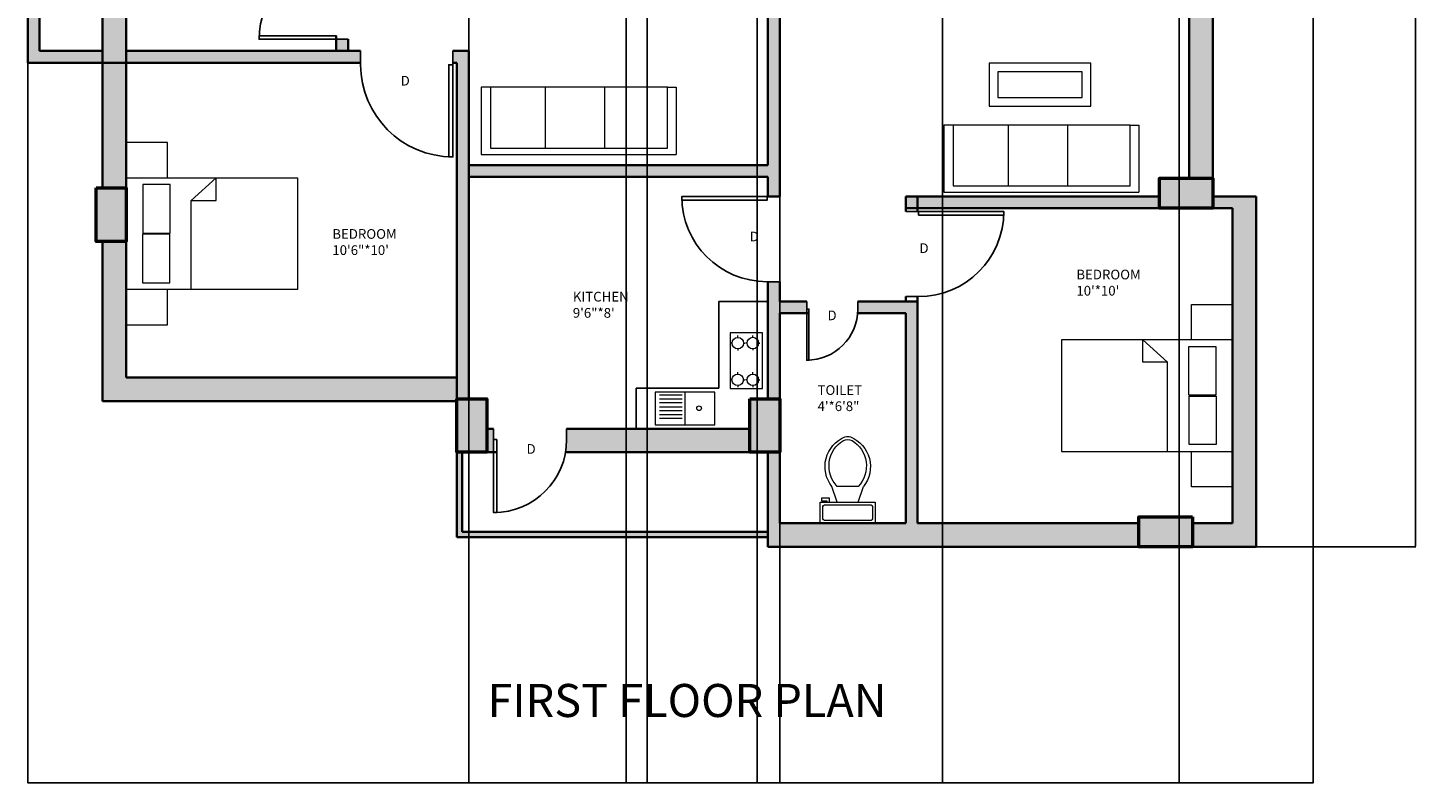
# Model space of a CAD drawing. Units: inches. Extents: x 1998 to 2588, y 1139 to 1977.
# Tile 1 of 134: x 2059 to 2588, y 1139 to 1427. Entities that reach past the tile are written whole.
import ezdxf

# ---------------------------------------------------------------- set-up
doc = ezdxf.new("R2010")
doc.units = ezdxf.units.IN
for name, color, linetype, lineweight in [('A-ANNO-DIMS', 2, 'Continuous', 18), ('A-ANNO-TITL', 7, 'Continuous', 35), ('A-AREA-IDEN', 7, 'Continuous', 18), ('A-COLS-PATT', 250, 'Continuous', 13), ('A-DOOR-IDEN', 7, 'Continuous', 18), ('A-EQPM', 21, 'Continuous', 18), ('A-FLOR-CASE', 32, 'Continuous', 25), ('A-FLOR-FIXT', 9, 'Continuous', 18), ('A-WALL-PATT', 252, 'Continuous', 13), ('COLUMN', 10, 'Continuous', 50), ('DOOR', 52, 'Continuous', 25), ('FUR', 21, 'Continuous', 18), ('WALL', 200, 'Continuous', 35)]:
    doc.layers.add(name, color=color, linetype=linetype, lineweight=lineweight)
doc.styles.get("Standard").update_dxf_attribs({"font": 'arial.ttf'})
doc.dimstyles.get("Standard").update_dxf_attribs({"dimtxt": 0.18, "dimasz": 0.18, "dimexe": 0.18, "dimexo": 0.0625, "dimgap": 0.09, "dimtad": 0, "dimtih": 1, "dimtoh": 1, "dimdec": 4, "dimzin": 0, "dimdsep": 46, "dimtxsty": 'Standard', "dimcen": 0.09, "dimadec": 0, "dimazin": 0, "dimtfac": 1, "dimtdec": 4, "dimtofl": 0, "dimtmove": 0, "dimatfit": 3, "dimfxl": 1, "dimtolj": 1, "dimtzin": 0, "dimarcsym": 0})

# ---------------------------------------------------------------- blocks, each defined once
blk = doc.blocks.new('*U2')
for p, q in [((0, 0), (0, -6)), ((40, 0), (40, -6))]:
    blk.add_line(p, q)
blk.add_lwpolyline([(0, 0), (0, 40), (1.75, 40), (1.75, 0)], close=True)
blk.add_arc((0, 0), 40, 0, 90)
blk = doc.blocks.new('*U4')
for p, q in [((9.5, -6), (9.5, -2)), ((-10, -8.5), (-8, -8.5)), ((-10, -9.5), (-10, -8.5)), ((-7, -9.5), (-10, -9.5)), ((-8, -8.5), (-8, -8)), ((-7, -8), (-7, -9.5)), ((-4, -8), (-6, -14)), ((4, -8), (6, -14)), ((4, -14), (-4, -14))]:
    blk.add_line(p, q)
blk.add_lwpolyline([(10.5, -8), (10.5, 0), (-10.5, 0), (-10.5, -8)], close=True)
for points in [[(-9.5, -2), (-9.5, -6)], [(8.5, -1), (-8.5, -1)], [(-8.5, -7), (8.5, -7)]]:
    blk.add_lwpolyline(points)
for centre, radius, start, end in [((-8.62, -1.88), 0.884, 81.8699, 188.1301), ((8.62, -1.88), 0.884, 351.8699, 98.1301), ((-8.62, -6.12), 0.884, 171.8699, 278.1301), ((8.62, -6.12), 0.884, 261.8699, 8.1301), ((3.52, -21.58), 12.17, 141.4691, 247.9714), ((4.2, -21.82), 11.33, 136.3677, 238.9468), ((-3.52, -21.58), 12.17, 292.0284, 38.5307), ((-4.2, -21.82), 11.33, 301.053, 43.6321), ((0, -27.88), 4, 245.7318, 294.2682), ((0, -29), 4, 254.8605, 285.1395)]:
    blk.add_arc(centre, radius, start, end)
blk = doc.blocks.new('BED-WITH-NIGHTSTANDS')
for p, q in [((34.22, 56), (24.8, 47.44)), ((34.22, 47.44), (34.22, 56)), ((24.8, 13.42), (24.8, 47.44)), ((24.8, 47.44), (34.22, 47.44))]:
    blk.add_line(p, q)
for points in [[(0, 56), (15.7, 56), (15.7, 69.42), (0, 69.42)], [(0, 56), (65.22, 56), (65.22, 13.42), (0, 13.42)], [(6.37, 34.93), (16.73, 34.93), (16.73, 53.45), (6.37, 53.45)], [(6.25, 16.05), (16.6, 16.05), (16.6, 34.57), (6.25, 34.57)], [(0, 0), (15.7, 0), (15.7, 13.42), (0, 13.42)]]:
    blk.add_lwpolyline(points, close=True)
blk = doc.blocks.new('SOFA-THREE-SEAT')
for p, q in [((3.6, 25.61), (0, 25.61)), ((0, 25.61), (0, 0)), ((24.45, 25.61), (24.45, 2.42)), ((47.08, 25.61), (47.08, 2.42)), ((71.01, 25.61), (74.34, 25.61)), ((74.34, 25.61), (74.34, 0)), ((0, 0), (74.34, 0))]:
    blk.add_line(p, q)
blk.add_lwpolyline([(3.6, 2.42), (71.01, 2.42), (71.01, 25.61), (3.6, 25.61)], close=True)
blk = doc.blocks.new('TABLE-COFFEE')
for points in [[(0, 0), (38.73, 0), (38.73, 16.33), (0, 16.33)], [(3.28, 3.28), (35.45, 3.28), (35.45, 13.05), (3.28, 13.05)]]:
    blk.add_lwpolyline(points, close=True)
blk = doc.blocks.new('*D23')
at = {"layer": 'A-ANNO-DIMS', "color": 0, "lineweight": -2, "transparency": 16777216}
for p, q in [((2549.18, 1476.17), (2549.18, 1138.6)), ((2059.47, 1413.17), (2059.47, 1138.6)), ((2059.65, 1138.78), (2303.93, 1138.78)), ((2549, 1138.78), (2304.72, 1138.78))]:
    blk.add_line(p, q, dxfattribs=at)
at = {"layer": 'A-ANNO-DIMS', "color": 0, "transparency": 16777216}
for points in [[(2059.65, 1138.81), (2059.65, 1138.75), (2059.47, 1138.78)], [(2549, 1138.81), (2549, 1138.75), (2549.18, 1138.78)]]:
    blk.add_solid(points, dxfattribs=at)
at = {"layer": 'Defpoints', "color": 0, "transparency": 16777216}
for p in [(2549.18, 1476.23), (2059.47, 1413.23), (2549.18, 1138.78)]:
    blk.add_point(p, dxfattribs=at)
at = {"layer": 'A-ANNO-DIMS', "color": 0, "transparency": 16777216, "insert": (2304.33, 1138.78), "char_height": 0.18, "attachment_point": 5}
blk.add_mtext('\\A1;489.7', dxfattribs=at)
blk = doc.blocks.new('*D24')
at = {"layer": 'A-ANNO-DIMS', "color": 0, "lineweight": -2, "transparency": 16777216}
for p, q in [((2398.54, 1911.23), (2588.31, 1911.23)), ((2588.13, 1911.05), (2588.13, 1570.16)), ((2588.13, 1228.91), (2588.13, 1569.8)), ((2527.54, 1228.73), (2588.31, 1228.73))]:
    blk.add_line(p, q, dxfattribs=at)
at = {"layer": 'A-ANNO-DIMS', "color": 0, "transparency": 16777216}
for points in [[(2588.1, 1911.05), (2588.16, 1911.05), (2588.13, 1911.23)], [(2588.1, 1228.91), (2588.16, 1228.91), (2588.13, 1228.73)]]:
    blk.add_solid(points, dxfattribs=at)
at = {"layer": 'Defpoints', "color": 0, "transparency": 16777216}
for p in [(2398.47, 1911.23), (2588.13, 1911.23), (2527.47, 1228.73)]:
    blk.add_point(p, dxfattribs=at)
at = {"layer": 'A-ANNO-DIMS', "color": 0, "transparency": 16777216, "insert": (2588.13, 1569.98), "char_height": 0.18, "attachment_point": 5}
blk.add_mtext('\\A1;682.5', dxfattribs=at)
blk = doc.blocks.new('*D33')
at = {"layer": 'A-ANNO-DIMS', "color": 0, "lineweight": -2, "transparency": 16777216}
for p, q in [((2407.97, 1480.67), (2407.97, 1138.6)), ((2498.18, 1480.67), (2498.18, 1138.6)), ((2408.15, 1138.78), (2452.75, 1138.78)), ((2498, 1138.78), (2453.4, 1138.78))]:
    blk.add_line(p, q, dxfattribs=at)
at = {"layer": 'A-ANNO-DIMS', "color": 0, "transparency": 16777216}
for points in [[(2408.15, 1138.81), (2408.15, 1138.75), (2407.97, 1138.78)], [(2498, 1138.81), (2498, 1138.75), (2498.18, 1138.78)]]:
    blk.add_solid(points, dxfattribs=at)
at = {"layer": 'Defpoints', "color": 0, "transparency": 16777216}
for p in [(2407.97, 1480.73), (2498.18, 1480.73), (2498.18, 1138.78)]:
    blk.add_point(p, dxfattribs=at)
at = {"layer": 'A-ANNO-DIMS', "color": 0, "transparency": 16777216, "insert": (2453.08, 1138.78), "char_height": 0.18, "attachment_point": 5}
blk.add_mtext('\\A1;90.2', dxfattribs=at)
blk = doc.blocks.new('*D41')
at = {"layer": 'A-ANNO-DIMS', "color": 0, "lineweight": -2, "transparency": 16777216}
for p, q in [((2227.47, 1588.67), (2227.47, 1138.6)), ((2287.47, 1588.67), (2287.47, 1138.6)), ((2227.65, 1138.78), (2257.25, 1138.78)), ((2287.29, 1138.78), (2257.69, 1138.78))]:
    blk.add_line(p, q, dxfattribs=at)
at = {"layer": 'A-ANNO-DIMS', "color": 0, "transparency": 16777216}
for points in [[(2227.65, 1138.81), (2227.65, 1138.75), (2227.47, 1138.78)], [(2287.29, 1138.81), (2287.29, 1138.75), (2287.47, 1138.78)]]:
    blk.add_solid(points, dxfattribs=at)
at = {"layer": 'Defpoints', "color": 0, "transparency": 16777216}
for p in [(2227.47, 1588.73), (2287.47, 1588.73), (2287.47, 1138.78)]:
    blk.add_point(p, dxfattribs=at)
at = {"layer": 'A-ANNO-DIMS', "color": 0, "transparency": 16777216, "insert": (2257.47, 1138.78), "char_height": 0.18, "attachment_point": 5}
blk.add_mtext('\\A1;60', dxfattribs=at)
blk = doc.blocks.new('*D43')
at = {"layer": 'A-ANNO-DIMS', "color": 0, "lineweight": -2, "transparency": 16777216}
for p, q in [((2407.97, 1594.67), (2407.97, 1138.6)), ((2345.97, 1588.67), (2345.97, 1138.6)), ((2346.15, 1138.78), (2376.75, 1138.78)), ((2407.79, 1138.78), (2377.19, 1138.78))]:
    blk.add_line(p, q, dxfattribs=at)
at = {"layer": 'A-ANNO-DIMS', "color": 0, "transparency": 16777216}
for points in [[(2346.15, 1138.81), (2346.15, 1138.75), (2345.97, 1138.78)], [(2407.79, 1138.81), (2407.79, 1138.75), (2407.97, 1138.78)]]:
    blk.add_solid(points, dxfattribs=at)
at = {"layer": 'Defpoints', "color": 0, "transparency": 16777216}
for p in [(2407.97, 1594.73), (2345.97, 1588.73), (2407.97, 1138.78)]:
    blk.add_point(p, dxfattribs=at)
at = {"layer": 'A-ANNO-DIMS', "color": 0, "transparency": 16777216, "insert": (2376.97, 1138.78), "char_height": 0.18, "attachment_point": 5}
blk.add_mtext('\\A1;62', dxfattribs=at)
blk = doc.blocks.new('*D44')
at = {"layer": 'A-ANNO-DIMS', "color": 0, "lineweight": -2, "transparency": 16777216}
for p, q in [((2295.41, 1588.67), (2295.41, 1138.6)), ((2337.29, 1588.67), (2337.29, 1138.6)), ((2295.59, 1138.78), (2315.95, 1138.78)), ((2337.11, 1138.78), (2316.75, 1138.78))]:
    blk.add_line(p, q, dxfattribs=at)
at = {"layer": 'A-ANNO-DIMS', "color": 0, "transparency": 16777216}
for points in [[(2295.59, 1138.81), (2295.59, 1138.75), (2295.41, 1138.78)], [(2337.11, 1138.81), (2337.11, 1138.75), (2337.29, 1138.78)]]:
    blk.add_solid(points, dxfattribs=at)
at = {"layer": 'Defpoints', "color": 0, "transparency": 16777216}
for p in [(2295.41, 1588.73), (2337.29, 1588.73), (2337.29, 1138.78)]:
    blk.add_point(p, dxfattribs=at)
at = {"layer": 'A-ANNO-DIMS', "color": 0, "transparency": 16777216, "insert": (2316.35, 1138.78), "char_height": 0.18, "attachment_point": 5}
blk.add_mtext('\\A1;41.87', dxfattribs=at)

msp = doc.modelspace()

# ---------------------------------------------------------------- hatches: boundary and pattern name
at = {"layer": 'A-COLS-PATT'}
h = msp.add_hatch(color=256, dxfattribs=at)
h.dxf.hatch_style = 1
h.paths.add_polyline_path([(2099.4125, 1888.7324), (2087.9729, 1888.7324), (2087.9729, 1868.3278), (2099.4125, 1868.3278)])
h.paths.add_polyline_path([(2234.4125, 1888.7324), (2222.9729, 1888.7324), (2222.9729, 1868.3278), (2234.4125, 1868.3278)])
h.paths.add_polyline_path([(2341.4729, 1886.637), (2330.0332, 1886.637), (2330.0332, 1866.2324), (2341.4729, 1866.2324)])
h.paths.add_polyline_path([(2507.8006, 1882.7324), (2487.396, 1882.7324), (2487.396, 1871.2927), (2507.8006, 1871.2927)])
h.paths.add_polyline_path([(2510.9729, 1766.672), (2490.5682, 1766.672), (2490.5682, 1755.2324), (2510.9729, 1755.2324)])
h.paths.add_polyline_path([(2345.9729, 1759.7324), (2334.5332, 1759.7324), (2334.5332, 1739.3278), (2345.9729, 1739.3278)])
h.paths.add_polyline_path([(2234.4125, 1774.3318), (2222.9729, 1774.3318), (2222.9729, 1753.9272), (2234.4125, 1753.9272)])
h.paths.add_polyline_path([(2099.4125, 1775.637), (2087.9729, 1775.637), (2087.9729, 1755.2324), (2099.4125, 1755.2324)])
h.paths.add_polyline_path([(2098.0956, 1593.7241), (2077.691, 1593.7241), (2077.691, 1582.2845), (2098.0956, 1582.2845)])
h.paths.add_polyline_path([(2227.4729, 1604.637), (2216.0332, 1604.637), (2216.0332, 1584.2324), (2227.4729, 1584.2324)])
h.paths.add_polyline_path([(2345.9729, 1647.5211), (2334.5332, 1647.5211), (2334.5332, 1627.1165), (2345.9729, 1627.1165)])
h.paths.add_polyline_path([(2522.3775, 1641.2324), (2501.9729, 1641.2324), (2501.9729, 1629.7927), (2522.3775, 1629.7927)])
h.paths.add_polyline_path([(2522.3775, 1480.7324), (2501.9729, 1480.7324), (2501.9729, 1469.2927), (2522.3775, 1469.2927)])
h.paths.add_polyline_path([(2345.9729, 1488.5616), (2334.5332, 1488.5616), (2334.5332, 1468.1569), (2345.9729, 1468.1569)])
h.paths.add_polyline_path([(2234.4125, 1486.137), (2227.4729, 1486.137), (2227.4729, 1465.7324), (2234.4125, 1465.7324)])
h.paths.add_polyline_path([(2227.4729, 1486.137), (2222.9729, 1486.137), (2222.9729, 1465.7324), (2227.4729, 1465.7324)])
h.paths.add_polyline_path([(2108.3775, 1470.2324), (2087.9729, 1470.2324), (2087.9729, 1458.7927), (2108.3775, 1458.7927)])
h.paths.add_polyline_path([(2096.9729, 1365.5012), (2087.9729, 1365.5012), (2087.9729, 1345.0966), (2096.9729, 1345.0966)])
h.paths.add_polyline_path([(2087.9729, 1365.5012), (2085.5332, 1365.5012), (2085.5332, 1345.0966), (2087.9729, 1345.0966)])
h.paths.add_polyline_path([(2234.4125, 1285.137), (2222.9729, 1285.137), (2222.9729, 1264.7324), (2234.4125, 1264.7324)])
h.paths.add_polyline_path([(2345.9729, 1285.137), (2334.5332, 1285.137), (2334.5332, 1264.7324), (2345.9729, 1264.7324)])
h.paths.add_polyline_path([(2503.1458, 1240.172), (2482.7412, 1240.172), (2482.7412, 1228.7324), (2503.1458, 1228.7324)])
h.paths.add_polyline_path([(2510.9729, 1369.172), (2490.5682, 1369.172), (2490.5682, 1357.7324), (2510.9729, 1357.7324)])
at = {"layer": 'A-WALL-PATT'}
h = msp.add_hatch(color=256, dxfattribs=at)
h.dxf.hatch_style = 1
h.paths.add_polyline_path([(2227.4729, 1911.2324), (2222.9729, 1911.2324), (2222.9729, 1888.7324), (2227.4729, 1888.7324)])
h.paths.add_polyline_path([(2236.4493, 1870.3636), (2236.4493, 1875.2324), (2234.4125, 1875.2324), (2234.4125, 1868.3278), (2227.4729, 1868.3278), (2227.4729, 1866.2324), (2236.4493, 1866.2324)])
h.paths.add_polyline_path([(2330.0332, 1875.2324), (2263.9907, 1875.2324), (2263.9907, 1866.2324), (2330.0332, 1866.2324)])
h.paths.add_polyline_path([(2345.9729, 1906.7324), (2393.9729, 1906.7324), (2393.9729, 1882.7324), (2345.9729, 1882.7324), (2345.9729, 1878.2324), (2393.9729, 1878.2324), (2398.4729, 1878.2324), (2398.4729, 1882.7324), (2398.4729, 1911.2324), (2345.9729, 1911.2324), (2341.4729, 1911.2324), (2341.4729, 1866.2324), (2341.4729, 1790.0412), (2345.9729, 1790.0412), (2345.9729, 1875.2324)])
h.paths.add_polyline_path([(2398.4729, 1878.2324), (2393.9729, 1878.2324), (2393.9729, 1798.2324), (2393.9729, 1793.7324), (2398.4729, 1793.7324)], flags=17)
h.paths.add_polyline_path([(2393.9729, 1798.2324), (2375.7311, 1798.2324, -0.00596797), (2375.7384, 1797.6146), (2375.7384, 1793.7324), (2393.9729, 1793.7324)], flags=17)
h.paths.add_polyline_path([(2349.8569, 1797.6146), (2349.8569, 1798.2324), (2345.9729, 1798.2324), (2345.9729, 1793.7324), (2349.8569, 1793.7324)], flags=17)
h.paths.add_polyline_path([(2398.4729, 1793.7324), (2393.9729, 1793.7324), (2393.9729, 1790.0412), (2398.4729, 1790.0412)], flags=17)
h.paths.add_polyline_path([(2527.4729, 1882.7324), (2507.8006, 1882.7324), (2507.8006, 1878.2324), (2518.4729, 1878.2324), (2518.4729, 1759.7324), (2510.9729, 1759.7324), (2510.9729, 1755.2324), (2527.4729, 1755.2324)])
h.paths.add_polyline_path([(2487.396, 1882.7324), (2398.4729, 1882.7324), (2398.4729, 1878.2324), (2487.396, 1878.2324)])
h.paths.add_polyline_path([(2490.5682, 1759.7324), (2345.9729, 1759.7324), (2345.9729, 1755.2324), (2490.5682, 1755.2324)])
h.paths.add_polyline_path([(2398.4729, 1760.5844), (2398.3914, 1760.5844), (2393.9729, 1760.5844), (2393.9729, 1759.7324), (2398.4729, 1759.7324)])
h.paths.add_polyline_path([(2334.5332, 1759.7324), (2234.4125, 1759.7324), (2234.4125, 1755.2324), (2334.5332, 1755.2324)])
h.paths.add_polyline_path([(2345.9729, 1760.5844), (2341.5543, 1760.5844), (2341.4729, 1760.5844), (2341.4729, 1759.7324), (2345.9729, 1759.7324)])
h.paths.add_polyline_path([(2222.9729, 1759.7324), (2221.7204, 1759.7324), (2221.7204, 1755.2324), (2222.9729, 1755.2324)])
h.paths.add_polyline_path([(2061.4729, 1702.7324), (2059.4729, 1702.7324), (2059.4729, 1584.2324), (2061.4729, 1584.2324)])
h.paths.add_polyline_path([(2061.4729, 1584.2324), (2059.4729, 1584.2324), (2059.4729, 1470.2324), (2061.4729, 1470.2324)])
h.paths.add_polyline_path([(2510.9729, 1469.2927), (2501.9729, 1469.2927), (2501.9729, 1369.172), (2510.9729, 1369.172)])
h.paths.add_polyline_path([(2227.4729, 1369.7324), (2227.4729, 1417.7324), (2221.4126, 1417.7324), (2221.4126, 1413.2324), (2222.9729, 1413.2324), (2222.9729, 1293.2324), (2222.9729, 1285.137), (2227.4729, 1285.137)])
h = msp.add_hatch(color=256, dxfattribs=at)
h.dxf.hatch_style = 1
h.paths.add_polyline_path([(2222.9729, 1888.7324), (2099.4125, 1888.7324), (2099.4125, 1879.7324), (2222.9729, 1879.7324)])
h.paths.add_polyline_path([(2096.9729, 1868.3278), (2087.9729, 1868.3278), (2087.9729, 1775.637), (2096.9729, 1775.637)])
h.paths.add_polyline_path([(2227.4729, 1868.3278), (2222.9729, 1868.3278), (2222.9729, 1774.3318), (2227.4729, 1774.3318)])
h.paths.add_polyline_path([(2188.3019, 1759.7324), (2138.6074, 1759.7324), (2099.4125, 1759.7324), (2099.4125, 1755.2324), (2176.9729, 1755.2324), (2188.3019, 1755.2324)])
h.paths.add_polyline_path([(2087.9729, 1759.7324), (2059.4729, 1759.7324), (2059.4729, 1702.7324), (2087.9729, 1702.7324), (2087.9729, 1707.2324), (2063.9729, 1707.2324), (2063.9729, 1755.2324), (2087.9729, 1755.2324)])
h.paths.add_polyline_path([(2096.9729, 1755.2324), (2087.9729, 1755.2324), (2087.9729, 1707.2324), (2096.9729, 1707.2324)])
h.paths.add_polyline_path([(2187.0461, 1707.2324), (2105.9729, 1707.2324), (2096.9729, 1707.2324), (2087.9729, 1707.2324), (2087.9729, 1702.7324), (2105.9729, 1702.7324), (2114.9729, 1702.7324), (2187.0461, 1702.7324)])
h.paths.add_polyline_path([(2181.4729, 1719.2028), (2176.9729, 1719.2028), (2176.9729, 1707.2324), (2181.4729, 1707.2324)])
h.paths.add_polyline_path([(2216.0332, 1588.7324), (2114.9729, 1588.7324), (2105.9729, 1588.7324), (2105.9729, 1584.2324), (2216.0332, 1584.2324)])
h.paths.add_polyline_path([(2077.691, 1588.7324), (2061.4729, 1588.7324), (2061.4729, 1584.2324), (2077.691, 1584.2324)])
h.paths.add_polyline_path([(2105.9729, 1588.7324), (2098.0956, 1588.7324), (2098.0956, 1584.2324), (2105.9729, 1584.2324)])
h.paths.add_polyline_path([(2114.9729, 1596.2642), (2110.1012, 1596.2642), (2105.9729, 1596.2642), (2105.9729, 1588.7324), (2114.9729, 1588.7324)])
h.paths.add_polyline_path([(2114.9729, 1584.2324), (2105.9729, 1584.2324), (2105.9729, 1580.249), (2110.1012, 1580.249), (2114.9729, 1580.249)])
h.paths.add_polyline_path([(2114.9729, 1547.7716), (2110.1012, 1547.7716, -0.0318759), (2105.9729, 1548.035), (2105.9729, 1470.2324), (2108.3775, 1470.2324), (2108.3775, 1465.7324), (2186.2943, 1465.7324), (2186.2943, 1470.2324), (2114.9729, 1470.2324)])
h.paths.add_polyline_path([(2227.4729, 1584.2324), (2222.9729, 1584.2324), (2222.9729, 1486.137), (2227.4729, 1486.137)])
h.paths.add_polyline_path([(2295.4138, 1593.2324), (2227.4729, 1593.2324), (2227.4729, 1588.7324), (2295.4138, 1588.7324), (2295.4138, 1591.8729)])
h.paths.add_polyline_path([(2345.9729, 1627.1165), (2341.4729, 1627.1165), (2341.4729, 1593.2324), (2337.2869, 1593.2324), (2337.2869, 1591.8729), (2337.2869, 1588.7324), (2345.9729, 1588.7324)])
h.paths.add_polyline_path([(2291.9729, 1588.7324), (2287.4729, 1588.7324), (2287.4729, 1522.7324), (2291.9729, 1522.7324)])
h.paths.add_polyline_path([(2291.9729, 1522.7324), (2287.4729, 1522.7324), (2227.4729, 1522.7324), (2227.4729, 1518.2324), (2291.9729, 1518.2324)])
h.paths.add_polyline_path([(2295.7347, 1519.5919), (2295.7347, 1522.7324), (2291.9729, 1522.7324), (2291.9729, 1518.2324), (2295.7347, 1518.2324)])
h.paths.add_polyline_path([(2345.9729, 1522.7324), (2337.6078, 1522.7324), (2337.6078, 1519.5919), (2337.6078, 1518.2324), (2341.4729, 1518.2324), (2341.4729, 1488.5616), (2345.9729, 1488.5616)])
h.paths.add_polyline_path([(2345.9729, 1468.1569), (2341.4729, 1468.1569), (2341.4729, 1374.2324), (2227.4729, 1374.2324), (2227.4729, 1369.7324), (2345.9729, 1369.7324)])
h.paths.add_polyline_path([(2345.9729, 1369.7324), (2341.4729, 1369.7324), (2341.4729, 1362.2324), (2345.9729, 1362.2324)])
h.paths.add_polyline_path([(2345.9729, 1317.7324), (2345.9729, 1322.2324), (2341.4729, 1322.2324), (2341.4729, 1285.137), (2345.9729, 1285.137)], flags=17)
h.paths.add_polyline_path([(2356.2096, 1322.2324), (2345.9729, 1322.2324), (2345.9729, 1317.7324), (2356.2096, 1317.7324), (2356.2096, 1319.3088)], flags=17)
h.paths.add_polyline_path([(2393.9729, 1322.2324), (2375.6999, 1322.2324), (2375.6999, 1319.3088, -0.02024576), (2375.636, 1317.7324), (2393.9729, 1317.7324)], flags=17)
h.paths.add_polyline_path([(2398.4729, 1322.2324), (2393.9729, 1322.2324), (2393.9729, 1317.7324), (2393.9729, 1237.7324), (2345.9729, 1237.7324), (2345.9729, 1264.7324), (2341.4729, 1264.7324), (2341.4729, 1228.7324), (2393.9729, 1228.7324), (2482.7412, 1228.7324), (2482.7412, 1237.7324), (2398.4729, 1237.7324), (2398.4729, 1297.1029)])
h.paths.add_polyline_path([(2398.4729, 1362.2324), (2393.9729, 1362.2324), (2393.9729, 1357.7324), (2398.4729, 1357.7324)])
h.paths.add_polyline_path([(2345.9729, 1329.7549), (2341.4729, 1329.7549), (2341.4729, 1322.2324), (2345.9729, 1322.2324)])
h = msp.add_hatch(color=256, dxfattribs=at)
h.dxf.hatch_style = 1
h.paths.add_polyline_path([(2527.4729, 1362.2324), (2510.9729, 1362.2324), (2510.9729, 1357.7324), (2518.4729, 1357.7324), (2518.4729, 1237.7324), (2503.1458, 1237.7324), (2503.1458, 1228.7324), (2527.4729, 1228.7324)])
h.paths.add_polyline_path([(2490.5682, 1362.2324), (2398.4729, 1362.2324), (2398.4729, 1357.7324), (2490.5682, 1357.7324)])
h.paths.add_polyline_path([(2224.9729, 1264.7324), (2222.9729, 1264.7324), (2222.9729, 1232.4125), (2341.4729, 1232.4125), (2341.4729, 1234.4125), (2224.9729, 1234.4125)])
h.paths.add_polyline_path([(2334.5332, 1273.7324), (2264.7638, 1273.7324), (2264.7638, 1269.5611, -0.043659), (2264.3413, 1264.7324), (2334.5332, 1264.7324)])
h.paths.add_polyline_path([(2236.9551, 1273.7324), (2234.4125, 1273.7324), (2234.4125, 1264.7324), (2236.9551, 1264.7324), (2236.9551, 1269.5611)])
h.paths.add_polyline_path([(2222.9729, 1293.2324), (2096.9729, 1293.2324), (2096.9729, 1345.0966), (2087.9729, 1345.0966), (2087.9729, 1284.2324), (2222.9729, 1284.2324), (2222.9729, 1285.137)])
h.paths.add_polyline_path([(2096.9729, 1458.7927), (2087.9729, 1458.7927), (2087.9729, 1417.7324), (2087.9729, 1413.2324), (2096.9729, 1413.2324), (2096.9729, 1417.7324)])
h.paths.add_polyline_path([(2096.9729, 1413.2324), (2087.9729, 1413.2324), (2087.9729, 1365.5012), (2096.9729, 1365.5012), (2096.9729, 1369.3358)])
h.paths.add_polyline_path([(2186.2943, 1417.7324), (2138.6074, 1417.7324), (2096.9729, 1417.7324), (2096.9729, 1413.2324), (2138.6074, 1413.2324), (2186.2943, 1413.2324)])
h.paths.add_polyline_path([(2181.4729, 1465.7324), (2176.9729, 1465.7324), (2176.9729, 1451.6434), (2181.4729, 1451.6434)])
h.paths.add_polyline_path([(2181.4729, 1422.1664), (2176.9729, 1422.1664), (2176.9729, 1417.7324), (2181.4729, 1417.7324)])
h.paths.add_polyline_path([(2063.9729, 1465.7324), (2087.9729, 1465.7324), (2087.9729, 1470.2324), (2059.4729, 1470.2324), (2059.4729, 1413.2324), (2087.9729, 1413.2324), (2087.9729, 1417.7324), (2063.9729, 1417.7324)])
h.paths.add_polyline_path([(2181.4729, 1755.2324), (2176.9729, 1755.2324), (2176.9729, 1748.6798), (2177.0513, 1748.6798), (2181.4729, 1748.6798)])
h.paths.add_polyline_path([(2227.4729, 1707.2324), (2220.4647, 1707.2324), (2220.4647, 1702.7324), (2222.9729, 1702.7324), (2222.9729, 1604.637), (2227.4729, 1604.637)])
h.paths.add_polyline_path([(2114.9729, 1702.7324), (2105.9729, 1702.7324), (2105.9729, 1628.4781, -0.0318759), (2110.1012, 1628.7416), (2114.9729, 1628.7416)])
h.paths.add_polyline_path([(2345.9729, 1739.3278), (2341.4729, 1739.3278), (2341.4729, 1647.5211), (2345.9729, 1647.5211)])
h.paths.add_polyline_path([(2350.6273, 1641.2324), (2345.9729, 1641.2324), (2345.9729, 1636.7324), (2350.6273, 1636.7324), (2350.6273, 1639.8729)])
h.paths.add_polyline_path([(2501.9729, 1641.2324), (2407.9729, 1641.2324), (2392.5005, 1641.2324), (2392.5005, 1639.8729), (2392.5005, 1636.7324), (2501.9729, 1636.7324)])
h.paths.add_polyline_path([(2510.9729, 1755.2324), (2501.9729, 1755.2324), (2501.9729, 1641.2324), (2510.9729, 1641.2324)])
h.paths.add_polyline_path([(2549.1786, 1641.2324), (2522.3775, 1641.2324), (2522.3775, 1636.7324), (2540.1786, 1636.7324), (2540.1786, 1480.7324), (2522.3775, 1480.7324), (2522.3775, 1476.2324), (2549.1786, 1476.2324)])
h.paths.add_polyline_path([(2498.1786, 1594.7324), (2407.9729, 1594.7324), (2407.9729, 1585.7324), (2416.9729, 1585.7324), (2489.1786, 1585.7324), (2489.1786, 1531.7324), (2416.9729, 1531.7324), (2407.9729, 1531.7324), (2407.9729, 1522.7324), (2498.1786, 1522.7324)])
h.paths.add_polyline_path([(2351.6437, 1480.7324), (2345.9729, 1480.7324), (2345.9729, 1476.2324), (2351.6437, 1476.2324), (2351.6437, 1477.5919)])
h.paths.add_polyline_path([(2501.9729, 1480.7324), (2498.1786, 1480.7324), (2407.9729, 1480.7324), (2393.5168, 1480.7324), (2393.5168, 1477.5919), (2393.5168, 1476.2324), (2501.9729, 1476.2324)])

# ---------------------------------------------------------------- linework, layer by layer
at = {"layer": 'A-EQPM'}
for p, q in [((2329.972, 1308.5066), (2329.972, 1309.2199)), ((2335.6821, 1308.5582), (2335.6821, 1309.2715)), ((2327.7837, 1306.3183), (2327.2518, 1306.3183)), ((2329.972, 1304.13), (2329.972, 1303.5614)), ((2329.972, 1304.13), (2329.972, 1303.5614)), ((2332.1603, 1306.3183), (2332.7022, 1306.3183)), ((2333.4938, 1306.3699), (2332.9619, 1306.3699)), ((2335.6821, 1304.1816), (2335.6821, 1303.6131)), ((2337.8704, 1306.3699), (2338.4124, 1306.3699)), ((2337.8704, 1306.3699), (2338.4124, 1306.3699)), ((2327.7358, 1292.3788), (2327.2039, 1292.3788)), ((2329.9241, 1294.5672), (2329.9241, 1295.2804)), ((2332.1124, 1292.3788), (2332.6543, 1292.3788)), ((2333.4938, 1292.3788), (2332.9619, 1292.3788)), ((2335.6821, 1294.5672), (2335.6821, 1295.2804)), ((2337.8704, 1292.3788), (2338.4124, 1292.3788)), ((2329.9241, 1290.1905), (2329.9241, 1289.622)), ((2335.6821, 1290.1905), (2335.6821, 1289.622))]:
    msp.add_line(p, q, dxfattribs=at)
msp.add_lwpolyline([(2339.4255, 1310.3344), (2327.0929, 1310.3344), (2327.0929, 1289.0476), (2339.4255, 1289.0476)], close=True, dxfattribs=at)
for centre in [(2329.972, 1306.3183), (2335.6821, 1306.3699), (2329.9241, 1292.3788), (2335.6821, 1292.3788)]:
    msp.add_circle(centre, 2.1883, dxfattribs=at)
at = {"layer": 'A-FLOR-CASE'}
for p, q in [((2322.7926, 1289.176), (2322.7926, 1322.2479)), ((2322.7926, 1322.2479), (2341.4729, 1322.2324)), ((2291.2651, 1273.7324), (2291.2651, 1289.176)), ((2291.2651, 1289.176), (2322.7926, 1289.176))]:
    msp.add_line(p, q, dxfattribs=at)
at = {"layer": 'A-FLOR-FIXT'}
for p, q in [((2308.7726, 1286.4592), (2300.1816, 1286.4592)), ((2309.8841, 1275.2683), (2309.8841, 1287.6066)), ((2308.7726, 1284.9352), (2300.1816, 1284.9352)), ((2308.7726, 1283.5357), (2300.1816, 1283.5357)), ((2308.7726, 1281.9496), (2300.1816, 1281.9496)), ((2308.7726, 1280.5078), (2300.1816, 1280.5078)), ((2308.7726, 1279.0638), (2300.1816, 1279.0638)), ((2308.7726, 1277.6825), (2300.1816, 1277.6825))]:
    msp.add_line(p, q, dxfattribs=at)
msp.add_lwpolyline([(2321.2435, 1287.6066), (2298.5247, 1287.6066), (2298.5247, 1275.2683), (2321.2435, 1275.2683)], close=True, dxfattribs=at)
msp.add_circle((2315.2274, 1281.5165), 0.8708, dxfattribs=at)
at = {"layer": 'COLUMN'}
for points in [[(2085.5332, 1365.5012), (2096.9729, 1365.5012), (2096.9729, 1345.0966), (2085.5332, 1345.0966)], [(2510.9729, 1369.172), (2510.9729, 1357.7324), (2490.5682, 1357.7324), (2490.5682, 1369.172)], [(2222.9729, 1285.137), (2234.4125, 1285.137), (2234.4125, 1264.7324), (2222.9729, 1264.7324)], [(2334.5332, 1285.137), (2345.9729, 1285.137), (2345.9729, 1264.7324), (2334.5332, 1264.7324)], [(2503.1458, 1240.172), (2503.1458, 1228.7324), (2482.7412, 1228.7324), (2482.7412, 1240.172)]]:
    msp.add_lwpolyline(points, close=True, dxfattribs=at)
at = {"layer": 'FUR'}
for p, q in [((2131.1898, 1369.3358), (2121.7721, 1360.7722)), ((2131.1898, 1360.7722), (2131.1898, 1369.3358)), ((2121.7721, 1326.7602), (2121.7721, 1360.7722)), ((2121.7721, 1360.7722), (2131.1898, 1360.7722))]:
    msp.add_line(p, q, dxfattribs=at)
for points in [[(2096.9729, 1369.3358), (2112.672, 1369.3358), (2112.672, 1382.7606), (2096.9729, 1382.7606)], [(2096.9729, 1369.3358), (2162.1944, 1369.3358), (2162.1944, 1326.7602), (2096.9729, 1326.7602)], [(2103.3469, 1348.2655), (2113.6983, 1348.2655), (2113.6983, 1366.7857), (2103.3469, 1366.7857)], [(2103.2266, 1329.3845), (2113.5779, 1329.3845), (2113.5779, 1347.9047), (2103.2266, 1347.9047)], [(2096.9729, 1313.3355), (2112.672, 1313.3355), (2112.672, 1326.7602), (2096.9729, 1326.7602)]]:
    msp.add_lwpolyline(points, close=True, dxfattribs=at)
at = {"layer": 'WALL'}
for p, q in [((2345.9729, 1522.7324), (2345.9729, 1369.7324)), ((2501.9729, 1476.2324), (2501.9729, 1369.172)), ((2059.4729, 1413.2324), (2059.4729, 1470.2324)), ((2063.9729, 1417.7324), (2063.9729, 1465.7324)), ((2087.9729, 1417.7324), (2087.9729, 1470.2324)), ((2341.4729, 1468.1569), (2341.4729, 1374.2324)), ((2510.9729, 1469.2927), (2510.9729, 1357.7324)), ((2096.9729, 1417.7324), (2096.9729, 1458.7927)), ((2176.9729, 1417.7324), (2176.9729, 1423.4561)), ((2087.9729, 1417.7324), (2063.9729, 1417.7324)), ((2087.9729, 1365.5012), (2087.9729, 1417.7324)), ((2096.9729, 1417.7324), (2138.6074, 1417.7324)), ((2096.9729, 1413.2324), (2096.9729, 1417.7324)), ((2096.9729, 1417.7324), (2176.9729, 1417.7324)), ((2138.6074, 1417.7324), (2186.2943, 1417.7324)), ((2186.2943, 1417.7324), (2138.6074, 1417.7324)), ((2181.4729, 1417.7324), (2181.4729, 1422.1664)), ((2222.9729, 1417.7324), (2221.4126, 1417.7324)), ((2221.4126, 1417.7324), (2227.4729, 1417.7324)), ((2227.4729, 1417.7324), (2227.4729, 1285.137)), ((2087.9729, 1413.2324), (2059.4729, 1413.2324)), ((2087.9729, 1413.2324), (2096.9729, 1413.2324)), ((2096.9729, 1413.2324), (2138.6074, 1413.2324)), ((2096.9729, 1365.5012), (2096.9729, 1413.2324)), ((2138.6074, 1413.2324), (2186.2943, 1413.2324)), ((2221.4126, 1413.2324), (2222.9729, 1413.2324)), ((2222.9729, 1413.2324), (2222.9729, 1293.2324)), ((2341.4729, 1374.2324), (2227.4729, 1374.2324)), ((2222.9729, 1369.7324), (2222.9729, 1264.7324)), ((2341.4729, 1369.7324), (2227.4729, 1369.7324)), ((2227.4729, 1369.7324), (2227.4729, 1285.137)), ((2341.4729, 1362.2324), (2341.4729, 1369.7324)), ((2345.9729, 1362.2324), (2345.9729, 1369.7324)), ((2345.9729, 1362.2324), (2341.4729, 1362.2324)), ((2490.5682, 1362.2324), (2393.9729, 1362.2324)), ((2393.9729, 1356.5529), (2393.9729, 1362.2324)), ((2398.4729, 1357.7324), (2398.4729, 1362.2324)), ((2510.9729, 1362.2324), (2527.4729, 1362.2324)), ((2527.4729, 1362.2324), (2527.4729, 1228.7324)), ((2510.9729, 1357.7324), (2393.9729, 1357.7324)), ((2398.4729, 1357.7324), (2518.4729, 1357.7324)), ((2398.4729, 1356.5529), (2398.4729, 1357.7324)), ((2518.4729, 1357.7324), (2518.4729, 1237.7324)), ((2087.9729, 1284.2324), (2087.9729, 1345.0966)), ((2096.9729, 1293.2324), (2096.9729, 1345.0966)), ((2341.4729, 1329.7549), (2341.4729, 1322.2324)), ((2345.9729, 1329.7549), (2345.9729, 1322.2324)), ((2393.9729, 1322.2324), (2393.9729, 1324.0755)), ((2398.4729, 1322.2324), (2398.4729, 1324.0755)), ((2341.4729, 1285.137), (2341.4729, 1322.2324)), ((2345.9729, 1322.2324), (2356.2096, 1322.2324)), ((2345.9729, 1264.7324), (2345.9729, 1317.7324)), ((2345.9729, 1237.7324), (2345.9729, 1317.7324)), ((2345.9729, 1317.7324), (2357.0623, 1317.7324)), ((2375.636, 1317.7324), (2393.9729, 1317.7324)), ((2375.6999, 1322.2324), (2393.9729, 1322.2324)), ((2393.9729, 1322.2324), (2398.4729, 1322.2324)), ((2393.9729, 1317.7324), (2393.9729, 1237.7324)), ((2398.4729, 1322.2324), (2398.4729, 1297.1029)), ((2398.4729, 1237.7324), (2398.4729, 1297.1029)), ((2222.9729, 1293.2324), (2096.9729, 1293.2324)), ((2222.9729, 1284.2324), (2087.9729, 1284.2324)), ((2234.4125, 1273.7324), (2236.9551, 1273.7324)), ((2264.7638, 1273.7324), (2334.5332, 1273.7324)), ((2222.9729, 1264.7324), (2238.1718, 1264.7324)), ((2222.9729, 1264.7324), (2222.9729, 1232.4125)), ((2224.9729, 1264.7324), (2224.9729, 1234.4125)), ((2264.3413, 1264.7324), (2341.4729, 1264.7324)), ((2341.4729, 1264.7324), (2341.4729, 1228.7324)), ((2345.9729, 1237.7324), (2345.9729, 1264.7324)), ((2341.4729, 1234.4125), (2224.9729, 1234.4125)), ((2393.9729, 1237.7324), (2345.9729, 1237.7324)), ((2482.7412, 1237.7324), (2398.4729, 1237.7324)), ((2518.4729, 1237.7324), (2503.1458, 1237.7324)), ((2341.4729, 1232.4125), (2222.9729, 1232.4125)), ((2393.9729, 1228.7324), (2341.4729, 1228.7324)), ((2527.4729, 1228.7324), (2393.9729, 1228.7324))]:
    msp.add_line(p, q, dxfattribs=at)

# ---------------------------------------------------------------- block references
at = {"layer": 'A-FLOR-FIXT', "xscale": -1, "rotation": 180}
msp.add_blockref('*U4', (2371.8476, 1237.7324), dxfattribs=at)
at = {"layer": 'DOOR'}
for p, xscale, yscale, zscale, rotation in [((2177.0513, 1422.1664), 0.736924595324625, 0.736924595324625, 0.736924595324625, 90), ((2221.4126, 1412.4646), 0.877957807115804, 0.877957807115804, 0.877957807115804, 180), ((2341.1012, 1362.2324), -0.8119355758402486, 0.8119355758402486, 0.8119355758402486, 90), ((2398.8445, 1356.5529), 0.8119355758402486, 0.8119355758402486, 0.8119355758402486, 270), ((2356.2096, 1319.3088), -0.4872586433188619, 0.4872586433188619, 0.4872586433188619, 180), ((2236.9551, 1269.5611), -0.6952157385185675, 0.6952157385185675, 0.6952157385185675, 180)]:
    msp.add_blockref('*U2', p, dxfattribs=dict(at, xscale=xscale, yscale=yscale, zscale=zscale, rotation=rotation))
at = {"layer": 'FUR'}
for name, p in [('TABLE-COFFEE', (2425.703, 1396.674)), ('SOFA-THREE-SEAT', (2232.1703, 1378.242)), ('SOFA-THREE-SEAT', (2408.467, 1363.842))]:
    msp.add_blockref(name, p, dxfattribs=at)
at = {"layer": 'FUR', "extrusion": (0, 0, -1), "zscale": -1}
msp.add_blockref('BED-WITH-NIGHTSTANDS', (-2518.4727, 1251.6164), dxfattribs=at)

# ---------------------------------------------------------------- texts
at = {"layer": 'A-ANNO-TITL', "insert": (2234.6105, 1176.4432), "char_height": 12.596658, "attachment_point": 1}
msp.add_mtext_dynamic_manual_height_columns('FIRST FLOOR PLAN', width=1353.928333, gutter_width=62.9833, heights=[0], dxfattribs=at)
at = {"layer": 'A-AREA-IDEN', "char_height": 3.69875, "attachment_point": 1}
for s, insert in [('BEDROOM\\P10\'6"*10\'', (2175.4965, 1349.8074)), ("BEDROOM\\P10'*10'", (2458.956, 1334.3419)), ('KITCHEN\\P9\'6"*8\'', (2267.1254, 1325.9013)), ('TOILET\\P4\'*6\'8"', (2360.3514, 1290.3148))]:
    msp.add_mtext_dynamic_manual_height_columns(s, width=110.572713, gutter_width=18.4938, heights=[0], dxfattribs=dict(at, insert=insert))
at = {"layer": 'A-DOOR-IDEN', "char_height": 3.6988, "attachment_point": 1}
for insert in [(2201.5368, 1408.2195), (2334.5042, 1348.8366), (2399.1911, 1344.3924), (2364.1466, 1318.7775), (2249.4963, 1267.856)]:
    msp.add_mtext_dynamic_manual_height_columns('D', width=110.572713, gutter_width=18.4938, heights=[0], dxfattribs=dict(at, insert=insert))

# ---------------------------------------------------------------- dimensions: what is measured, and where the dimension line sits
at = {"layer": 'A-ANNO-DIMS'}
dim = msp.add_linear_dim(base=(2588.1286, 1911.2324), p1=(2527.4729, 1228.7324), p2=(2398.4729, 1911.2324), angle=90, dimstyle='Standard', override={"dimdec": 1, "dimlfac": 1, "dimrnd": 0, "dimzin": 0, "dimdsep": 46, "dimlunit": 2}, dxfattribs=at)
dim.commit()
dim.dimension.update_dxf_attribs({"geometry": '*D24', "text_midpoint": (2588.1286, 1569.9824)})
for base, p1, p2, override, picture, middle in [((2407.9729, 1138.7824), (2345.9729, 1588.7324), (2407.9729, 1594.7324), {"dimdec": 0, "dimlfac": 1, "dimrnd": 0, "dimzin": 0, "dimdsep": 46, "dimlunit": 2}, '*D43', (2376.9729, 1138.7824)), ((2287.4729, 1138.7824), (2227.4729, 1588.7324), (2287.4729, 1588.7324), {"dimdec": 0, "dimlfac": 1, "dimrnd": 0, "dimzin": 0, "dimdsep": 46, "dimlunit": 2}, '*D41', (2257.4729, 1138.7824)), ((2337.2869, 1138.7824), (2295.4138, 1588.7324), (2337.2869, 1588.7324), {"dimdec": 2, "dimlfac": 1, "dimrnd": 0, "dimzin": 0, "dimdsep": 46, "dimlunit": 2}, '*D44', (2316.3503, 1138.7824)), ((2549.1786, 1138.7824), (2059.4729, 1413.2324), (2549.1786, 1476.2324), {"dimdec": 1, "dimlfac": 1, "dimrnd": 0, "dimzin": 0, "dimdsep": 46, "dimlunit": 2}, '*D23', (2304.3257, 1138.7824)), ((2498.1786, 1138.7824), (2407.9729, 1480.7324), (2498.1786, 1480.7324), {"dimdec": 1, "dimlfac": 1, "dimrnd": 0, "dimzin": 0, "dimdsep": 46, "dimlunit": 2}, '*D33', (2453.0757, 1138.7824))]:
    dim = msp.add_linear_dim(base=base, p1=p1, p2=p2, dimstyle='Standard', override=override, dxfattribs=at)
    dim.commit()
    dim.dimension.update_dxf_attribs({"geometry": picture, "text_midpoint": middle})

doc.saveas('drawing.dxf')
